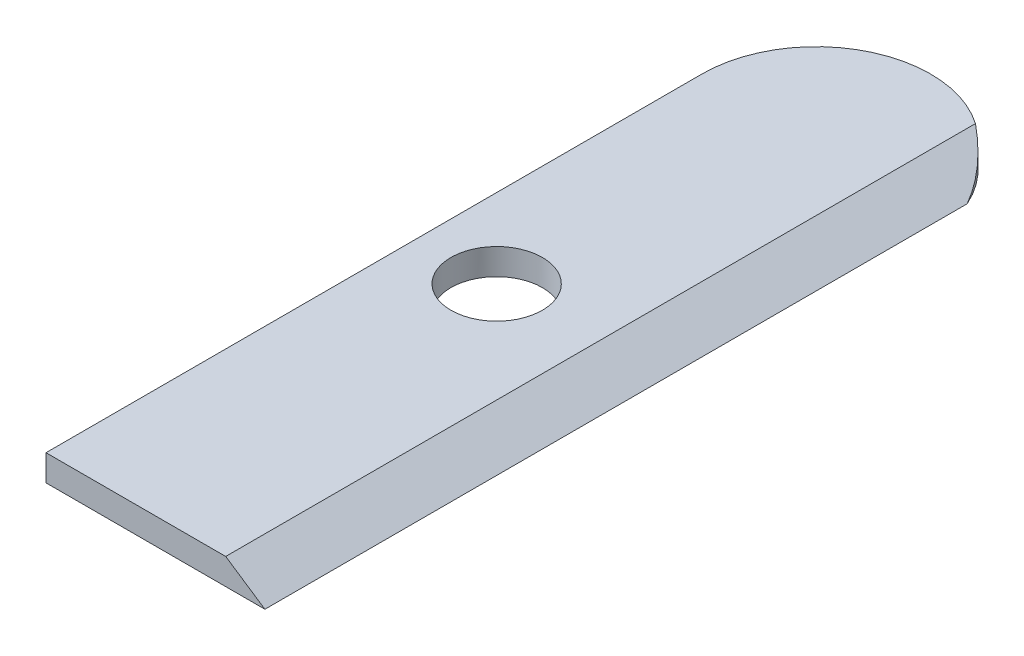
ISO-10303-21;
HEADER;
FILE_DESCRIPTION(('STEP AP214'),'2;1');
FILE_NAME('part.step','',(''),(''),'','','');
FILE_SCHEMA(('AUTOMOTIVE_DESIGN { 1 0 10303 214 1 1 1 1 }'));
ENDSEC;
DATA;
#1=APPLICATION_CONTEXT('core data for automotive mechanical design processes');
#2=APPLICATION_PROTOCOL_DEFINITION('international standard','automotive_design',2000,#1);
#3=PRODUCT_CONTEXT('',#1,'mechanical');
#4=PRODUCT('Part','Part','',(#3));
#5=PRODUCT_RELATED_PRODUCT_CATEGORY('part','',(#4));
#6=PRODUCT_DEFINITION_FORMATION('','',#4);
#7=PRODUCT_DEFINITION_CONTEXT('part definition',#1,'design');
#8=PRODUCT_DEFINITION('design','',#6,#7);
#9=PRODUCT_DEFINITION_SHAPE('','',#8);
#10=(LENGTH_UNIT() NAMED_UNIT(*) SI_UNIT(.MILLI.,.METRE.));
#11=(NAMED_UNIT(*) PLANE_ANGLE_UNIT() SI_UNIT($,.RADIAN.));
#12=(NAMED_UNIT(*) SI_UNIT($,.STERADIAN.) SOLID_ANGLE_UNIT());
#13=UNCERTAINTY_MEASURE_WITH_UNIT(LENGTH_MEASURE(1.E-05),#10,'distance_accuracy_value','');
#14=(GEOMETRIC_REPRESENTATION_CONTEXT(3) GLOBAL_UNCERTAINTY_ASSIGNED_CONTEXT((#13)) GLOBAL_UNIT_ASSIGNED_CONTEXT((#10,
#11,#12)) REPRESENTATION_CONTEXT('',''));
#15=CARTESIAN_POINT('',(0.,0.,0.));
#16=DIRECTION('',(0.,0.,1.));
#17=DIRECTION('',(1.,0.,0.));
#18=AXIS2_PLACEMENT_3D('',#15,#16,#17);
#19=CARTESIAN_POINT('',(-7.,0.8,0.));
#20=DIRECTION('',(1.,0.,0.));
#21=DIRECTION('',(0.,0.,-1.));
#22=AXIS2_PLACEMENT_3D('',#19,#20,#21);
#23=PLANE('',#22);
#24=DIRECTION('',(0.,0.,1.));
#25=VECTOR('',#24,1.);
#26=CARTESIAN_POINT('',(-7.,0.,0.));
#27=LINE('',#26,#25);
#28=CARTESIAN_POINT('',(-7.,0.,-20.0758212663472));
#29=VERTEX_POINT('',#28);
#30=CARTESIAN_POINT('',(-7.,0.,0.));
#31=VERTEX_POINT('',#30);
#32=EDGE_CURVE('E98',#29,#31,#27,.T.);
#33=ORIENTED_EDGE('',*,*,#32,.T.);
#34=DIRECTION('',(0.,-1.,0.));
#35=VECTOR('',#34,1.);
#36=CARTESIAN_POINT('',(-7.,0.8,0.));
#37=LINE('',#36,#35);
#38=CARTESIAN_POINT('',(-7.,0.8,0.));
#39=VERTEX_POINT('',#38);
#40=EDGE_CURVE('E83',#39,#31,#37,.T.);
#41=ORIENTED_EDGE('',*,*,#40,.F.);
#42=DIRECTION('',(0.,0.,1.));
#43=VECTOR('',#42,1.);
#44=CARTESIAN_POINT('',(-7.,0.8,0.));
#45=LINE('',#44,#43);
#46=CARTESIAN_POINT('',(-7.,0.8,-20.0758212663472));
#47=VERTEX_POINT('',#46);
#48=EDGE_CURVE('E87',#47,#39,#45,.T.);
#49=ORIENTED_EDGE('',*,*,#48,.F.);
#50=DIRECTION('',(0.,-1.,0.));
#51=VECTOR('',#50,1.);
#52=CARTESIAN_POINT('',(-7.,0.8,-20.0758212663472));
#53=LINE('',#52,#51);
#54=EDGE_CURVE('E99',#47,#29,#53,.T.);
#55=ORIENTED_EDGE('',*,*,#54,.T.);
#56=EDGE_LOOP('',(#33,#41,#49,#55));
#57=FACE_BOUND('',#56,.T.);
#58=ADVANCED_FACE('F41',(#57),#23,.F.);
#59=CARTESIAN_POINT('',(-0.300000000000004,0.8,0.));
#60=DIRECTION('',(0.,0.,-1.));
#61=DIRECTION('',(-1.,0.,0.));
#62=AXIS2_PLACEMENT_3D('',#59,#60,#61);
#63=PLANE('',#62);
#64=DIRECTION('',(1.,0.,0.));
#65=VECTOR('',#64,1.);
#66=CARTESIAN_POINT('',(-0.300000000000004,0.,0.));
#67=LINE('',#66,#65);
#68=CARTESIAN_POINT('',(-0.300000000000004,0.,0.));
#69=VERTEX_POINT('',#68);
#70=EDGE_CURVE('E115',#31,#69,#67,.T.);
#71=ORIENTED_EDGE('',*,*,#70,.T.);
#72=DIRECTION('',(0.832050294337845,-0.554700196225228,0.));
#73=VECTOR('',#72,1.);
#74=CARTESIAN_POINT('',(-1.50000000000001,0.799999999999998,0.));
#75=LINE('',#74,#73);
#76=CARTESIAN_POINT('',(-1.50000000000001,0.8,0.));
#77=VERTEX_POINT('',#76);
#78=EDGE_CURVE('E11',#69,#77,#75,.F.);
#79=ORIENTED_EDGE('',*,*,#78,.T.);
#80=DIRECTION('',(1.,0.,0.));
#81=VECTOR('',#80,1.);
#82=CARTESIAN_POINT('',(-0.300000000000004,0.8,0.));
#83=LINE('',#82,#81);
#84=EDGE_CURVE('E79',#39,#77,#83,.T.);
#85=ORIENTED_EDGE('',*,*,#84,.F.);
#86=ORIENTED_EDGE('',*,*,#40,.T.);
#87=EDGE_LOOP('',(#71,#79,#85,#86));
#88=FACE_BOUND('',#87,.T.);
#89=ADVANCED_FACE('F82',(#88),#63,.F.);
#90=CARTESIAN_POINT('',(-3.5,0.8,-20.0758212663472));
#91=DIRECTION('',(0.,-1.,0.));
#92=DIRECTION('',(0.,0.,-1.));
#93=AXIS2_PLACEMENT_3D('',#90,#91,#92);
#94=CYLINDRICAL_SURFACE('',#93,3.5);
#95=CARTESIAN_POINT('',(-3.5,0.8,-20.0758212663472));
#96=DIRECTION('',(0.,1.,0.));
#97=DIRECTION('',(0.,0.,-1.));
#98=AXIS2_PLACEMENT_3D('',#95,#96,#97);
#99=CIRCLE('',#98,3.5);
#100=CARTESIAN_POINT('',(-1.50000000000001,0.8,-22.9481025896162));
#101=VERTEX_POINT('',#100);
#102=EDGE_CURVE('E88',#101,#47,#99,.T.);
#103=ORIENTED_EDGE('',*,*,#102,.F.);
#104=CARTESIAN_POINT('',(-3.5,2.13333333333333,-20.0758212663472));
#105=DIRECTION('',(-0.554700196225228,-0.832050294337844,0.));
#106=DIRECTION('',(0.832050294337845,-0.554700196225228,0.));
#107=AXIS2_PLACEMENT_3D('',#104,#105,#106);
#108=ELLIPSE('',#107,4.20647648804132,3.5);
#109=CARTESIAN_POINT('',(-0.3,0.,-21.493565954223));
#110=VERTEX_POINT('',#109);
#111=EDGE_CURVE('E49',#101,#110,#108,.T.);
#112=ORIENTED_EDGE('',*,*,#111,.T.);
#113=CARTESIAN_POINT('',(-3.5,0.,-20.0758212663472));
#114=DIRECTION('',(0.,1.,0.));
#115=DIRECTION('',(0.,0.,-1.));
#116=AXIS2_PLACEMENT_3D('',#113,#114,#115);
#117=CIRCLE('',#116,3.5);
#118=EDGE_CURVE('E92',#110,#29,#117,.T.);
#119=ORIENTED_EDGE('',*,*,#118,.T.);
#120=ORIENTED_EDGE('',*,*,#54,.F.);
#121=EDGE_LOOP('',(#103,#112,#119,#120));
#122=FACE_BOUND('',#121,.T.);
#123=ADVANCED_FACE('F110',(#122),#94,.T.);
#124=CARTESIAN_POINT('',(-3.5,0.8,-20.0758212663472));
#125=DIRECTION('',(0.,-1.,0.));
#126=DIRECTION('',(0.,0.,-1.));
#127=AXIS2_PLACEMENT_3D('',#124,#125,#126);
#128=PLANE('',#127);
#129=CARTESIAN_POINT('',(-4.57873999743935,0.8,-11.3718951806636));
#130=DIRECTION('',(0.,1.,0.));
#131=DIRECTION('',(0.,0.,1.));
#132=AXIS2_PLACEMENT_3D('',#129,#130,#131);
#133=CIRCLE('',#132,1.4);
#134=CARTESIAN_POINT('',(-4.57873999743935,0.8,-9.9718951806636));
#135=VERTEX_POINT('',#134);
#136=EDGE_CURVE('E122',#135,#135,#133,.T.);
#137=ORIENTED_EDGE('',*,*,#136,.F.);
#138=EDGE_LOOP('',(#137));
#139=FACE_BOUND('',#138,.T.);
#140=ORIENTED_EDGE('',*,*,#84,.T.);
#141=DIRECTION('',(0.,0.,-1.));
#142=VECTOR('',#141,1.);
#143=CARTESIAN_POINT('',(-1.50000000000001,0.8,-20.0758212663472));
#144=LINE('',#143,#142);
#145=EDGE_CURVE('E97',#77,#101,#144,.T.);
#146=ORIENTED_EDGE('',*,*,#145,.T.);
#147=ORIENTED_EDGE('',*,*,#102,.T.);
#148=ORIENTED_EDGE('',*,*,#48,.T.);
#149=EDGE_LOOP('',(#140,#146,#147,#148));
#150=FACE_BOUND('',#149,.T.);
#151=ADVANCED_FACE('F89',(#139,#150),#128,.F.);
#152=CARTESIAN_POINT('',(-3.5,0.,-20.0758212663472));
#153=DIRECTION('',(0.,-1.,0.));
#154=DIRECTION('',(0.,0.,-1.));
#155=AXIS2_PLACEMENT_3D('',#152,#153,#154);
#156=PLANE('',#155);
#157=CARTESIAN_POINT('',(-4.57873999743935,0.,-11.3718951806636));
#158=DIRECTION('',(0.,-1.,0.));
#159=DIRECTION('',(0.,0.,-1.));
#160=AXIS2_PLACEMENT_3D('',#157,#158,#159);
#161=CIRCLE('',#160,1.4);
#162=CARTESIAN_POINT('',(-4.57873999743935,0.,-12.7718951806636));
#163=VERTEX_POINT('',#162);
#164=EDGE_CURVE('E120',#163,#163,#161,.T.);
#165=ORIENTED_EDGE('',*,*,#164,.F.);
#166=EDGE_LOOP('',(#165));
#167=FACE_BOUND('',#166,.T.);
#168=ORIENTED_EDGE('',*,*,#32,.F.);
#169=ORIENTED_EDGE('',*,*,#118,.F.);
#170=DIRECTION('',(0.,0.,-1.));
#171=VECTOR('',#170,1.);
#172=CARTESIAN_POINT('',(-0.300000000000004,0.,0.));
#173=LINE('',#172,#171);
#174=EDGE_CURVE('E112',#69,#110,#173,.T.);
#175=ORIENTED_EDGE('',*,*,#174,.F.);
#176=ORIENTED_EDGE('',*,*,#70,.F.);
#177=EDGE_LOOP('',(#168,#169,#175,#176));
#178=FACE_BOUND('',#177,.T.);
#179=ADVANCED_FACE('F109',(#167,#178),#156,.T.);
#180=CARTESIAN_POINT('',(-1.50000000000001,0.8,-20.0758212663472));
#181=DIRECTION('',(-0.554700196225228,-0.832050294337844,0.));
#182=DIRECTION('',(0.,0.,-1.));
#183=AXIS2_PLACEMENT_3D('',#180,#181,#182);
#184=PLANE('',#183);
#185=ORIENTED_EDGE('',*,*,#78,.F.);
#186=ORIENTED_EDGE('',*,*,#174,.T.);
#187=ORIENTED_EDGE('',*,*,#111,.F.);
#188=ORIENTED_EDGE('',*,*,#145,.F.);
#189=EDGE_LOOP('',(#185,#186,#187,#188));
#190=FACE_BOUND('',#189,.T.);
#191=ADVANCED_FACE('F42',(#190),#184,.F.);
#192=CARTESIAN_POINT('',(-4.57873999743935,0.8,-11.3718951806636));
#193=DIRECTION('',(0.,1.,0.));
#194=DIRECTION('',(0.,0.,1.));
#195=AXIS2_PLACEMENT_3D('',#192,#193,#194);
#196=CYLINDRICAL_SURFACE('',#195,1.4);
#197=ORIENTED_EDGE('',*,*,#164,.T.);
#198=EDGE_LOOP('',(#197));
#199=FACE_BOUND('',#198,.T.);
#200=ORIENTED_EDGE('',*,*,#136,.T.);
#201=EDGE_LOOP('',(#200));
#202=FACE_BOUND('',#201,.T.);
#203=ADVANCED_FACE('F121',(#199,#202),#196,.F.);
#204=CLOSED_SHELL('',(#58,#89,#123,#151,#179,#191,#203));
#205=MANIFOLD_SOLID_BREP('B2',#204);
#206=ADVANCED_BREP_SHAPE_REPRESENTATION('',(#18,#205),#14);
#207=SHAPE_DEFINITION_REPRESENTATION(#9,#206);
ENDSEC;
END-ISO-10303-21;
